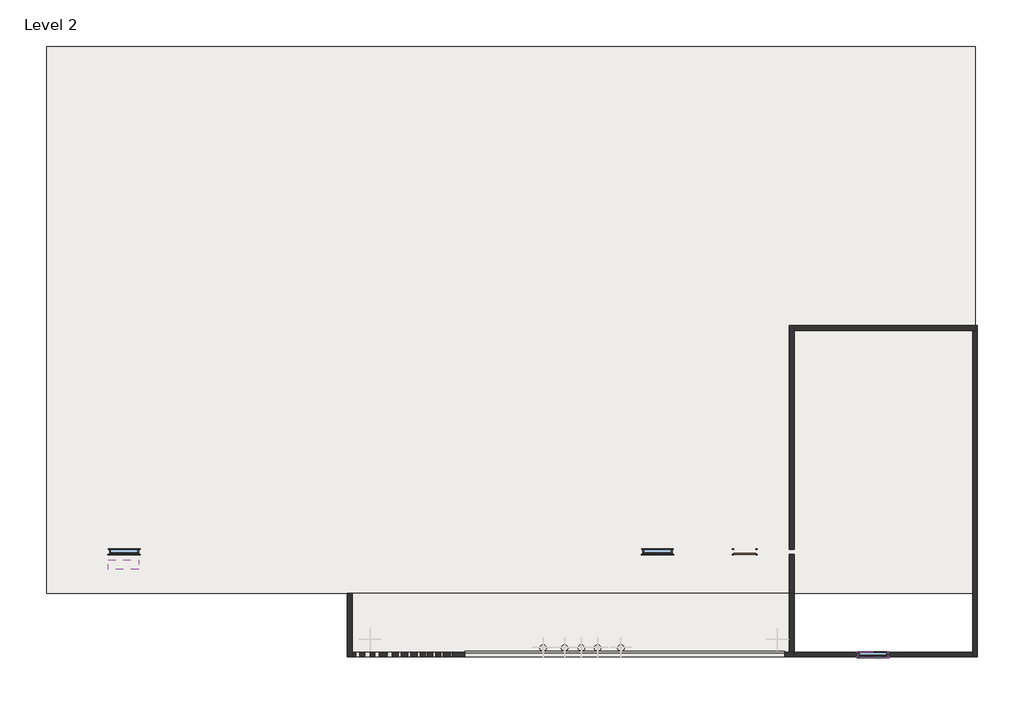
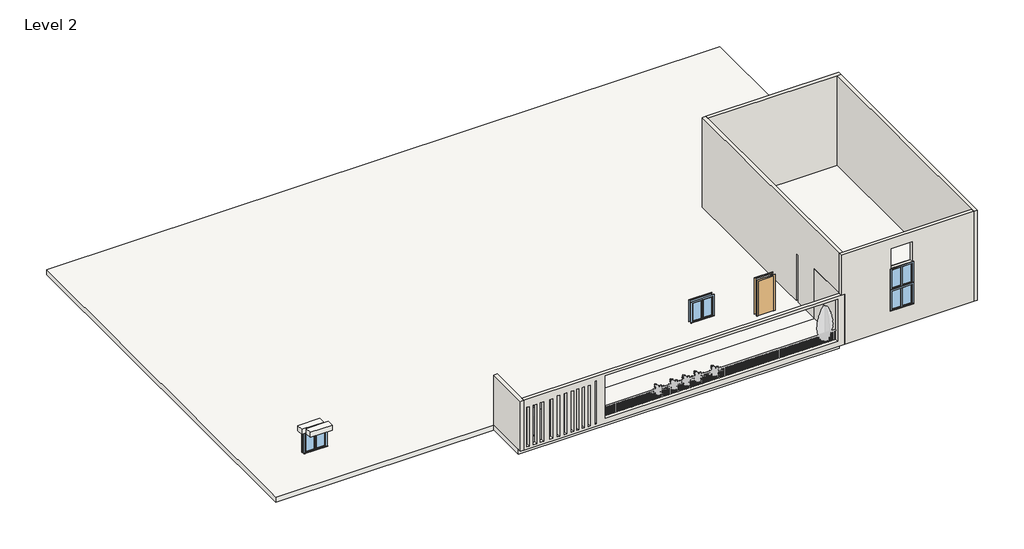
# One storey, part 1 of 2: 7 walls, 4 windows, 3 slabs, 1 door.
"""IFC4 building model written with IfcOpenShell, lengths in millimetres."""

from ifc_helpers import new_model, si_unit, frame, origin, place, context, project, spatial, polyline, outline, extrude, faceted_brep, transform, mapped, element, save
from components import door_54dd4da4, window_0862ab64

model = new_model("IFC4")

# Units and contexts
model_context = context("Model", 3, world=origin())
ifc_project = project(units=[si_unit("LENGTHUNIT", "METRE", prefix="MILLI")], contexts=[model_context])

# Site, building, storey
site = spatial("IfcSite", under=ifc_project)
building = spatial("IfcBuilding", under=site)
storey = spatial("IfcBuildingStorey", under=building, Name="Level 2", Elevation=3200.4)

# Door
placement = place(None, origin())
door_shape = door_54dd4da4(model_context)
element("IfcDoor", 1, ObjectType="Single-Flush : 36\" x 84\"", at=placement, inside=storey, context=model_context, shape_type="MappedRepresentation", body=[
    mapped(door_shape, transform((6933.8747398, -14818.870124, 3200.4), x_axis=(-1.0, 0.0, 0.0), y_axis=(0.0, -1.0, 0.0), z_axis=(0.0, 0.0, 1.0))),
])

# Slabs
element("IfcSlab", 2, ObjectType="Generic - 12\"", at=placement, inside=storey, context=model_context, shape_type="SweptSolid", body=[
    extrude(outline(polyline([(16585.8747398, 6378.5537948), (16585.8747398, -16555.9021378), (-22326.9252602, -16555.9021378), (-22326.9252602, 6378.5537948), (16585.8747398, 6378.5537948)])), frame((0.0, 0.0, 2895.6), z_axis=(0.0, 0.0, 1.0), x_axis=(1.0, 0.0, 0.0)), (0.0, 0.0, 1.0), 304.8),
])
element("IfcSlab", 3, ObjectType="Generic - 12\"", at=placement, inside=storey, context=model_context, shape_type="SweptSolid", body=[
    extrude(outline(polyline([(-18470.9809224, -15158.9638264), (-18470.9809224, -15539.9638264), (-19740.9809224, -15539.9638264), (-19740.9809224, -15158.9638264), (-18470.9809224, -15158.9638264)])), frame((0.0, 0.0, 5334.0), z_axis=(0.0, 0.0, 1.0), x_axis=(1.0, 0.0, 0.0)), (0.0, 0.0, 1.0), 304.8),
    extrude(outline(polyline([(-18710.9996532, -14717.270124), (-18710.9996532, -15098.270124), (-19980.9996532, -15098.270124), (-19980.9996532, -14717.270124), (-18710.9996532, -14717.270124)])), frame((0.0, 0.0, 5334.0), z_axis=(0.0, 0.0, 1.0), x_axis=(1.0, 0.0, 0.0)), (0.0, 0.0, 1.0), 304.8),
])
element("IfcSlab", 4, ObjectType="Generic - 12\"", at=placement, inside=storey, context=model_context, shape_type="SweptSolid", body=[
    extrude(outline(polyline([(8806.3760973, -16555.9021378), (8806.3760973, -19021.4462052), (-9727.8029191, -19021.4462052), (-9727.8029191, -16555.9021378), (8806.3760973, -16555.9021378)])), frame((0.0, 0.0, 2895.6), z_axis=(0.0, 0.0, 1.0), x_axis=(1.0, 0.0, 0.0)), (0.0, 0.0, 1.0), 304.8),
])

# Walls
element("IfcWall", 5, ObjectType="Generic - 8\"", at=placement, inside=storey, context=model_context, shape_type="Brep", body=[
    faceted_brep([(-9524.6029191, -19224.6462052, 3200.4), (-9524.6029191, -19021.4462052, 3200.4), (-9524.6029191, -16555.9021378, 3200.4), (-9524.6029191, -16555.9021378, 6248.4), (-9524.6029191, -19021.4462052, 6248.4), (-9524.6029191, -19224.6462052, 6248.4), (-9727.8029191, -19224.6462052, 3200.4), (-9727.8029191, -19224.6462052, 6248.4), (-9727.8029191, -16555.9021378, 6248.4), (-9727.8029191, -16555.9021378, 3200.4)], [[[0, 1, 2, 3, 4, 5]], [[6, 7, 8, 9]], [[2, 1, 0, 6, 9]], [[3, 2, 9, 8]], [[5, 4, 3, 8, 7]], [[0, 5, 7, 6]]]),
])
element("IfcWall", 6, ObjectType="Generic - 8\"", at=placement, inside=storey, context=model_context, shape_type="Brep", body=[
    faceted_brep([(9009.5760973, -19021.4462052, 3200.4), (8806.3760973, -19021.4462052, 3200.4), (-9524.6029191, -19021.4462052, 3200.4), (-9524.6029191, -19021.4462052, 6248.4), (8806.3760973, -19021.4462052, 6248.4), (9009.5760973, -19021.4462052, 6248.4), (8602.0331611, -19021.4462052, 6096.0), (-4809.1668389, -19021.4462052, 6096.0), (-4809.1668389, -19021.4462052, 3505.2), (8602.0331611, -19021.4462052, 3505.2), (-5331.1523958, -19021.4462052, 5990.1341587), (-5407.3523958, -19021.4462052, 5990.1341587), (-5407.3523958, -19021.4462052, 3348.5341587), (-5331.1523958, -19021.4462052, 3348.5341587), (-7464.3821742, -19021.4462052, 5843.7194015), (-7586.581963, -19021.4462052, 5843.7194015), (-7586.581963, -19021.4462052, 3348.5341587), (-7464.3821742, -19021.4462052, 3348.5341587), (-7057.0495448, -19021.4462052, 5843.7194015), (-7192.827088, -19021.4462052, 5843.7194015), (-7192.827088, -19021.4462052, 3348.5341587), (-7057.0495448, -19021.4462052, 3348.5341587), (-6656.5057926, -19021.4462052, 5843.7194015), (-6785.4944586, -19021.4462052, 5843.7194015), (-6785.4944586, -19021.4462052, 3348.5341587), (-6656.5057926, -19021.4462052, 3348.5341587), (-6364.5840749, -19021.4462052, 5843.7194015), (-6459.6283551, -19021.4462052, 5843.7194015), (-6459.6283551, -19021.4462052, 3348.5341587), (-6364.5840749, -19021.4462052, 3348.5341587), (-6025.1402171, -19021.4462052, 5843.7194015), (-6140.5511287, -19021.4462052, 5843.7194015), (-6140.5511287, -19021.4462052, 3348.5341587), (-6025.1402171, -19021.4462052, 3348.5341587), (-5699.2741136, -19021.4462052, 5843.7194015), (-5814.6850252, -19021.4462052, 5843.7194015), (-5814.6850252, -19021.4462052, 3348.5341587), (-5699.2741136, -19021.4462052, 3348.5341587), (-7844.559295, -19021.4462052, 5762.9412554), (-8041.4367325, -19021.4462052, 5762.9412554), (-8041.4367325, -19021.4462052, 3348.5341587), (-7844.559295, -19021.4462052, 3348.5341587), (-9209.1236034, -19021.4462052, 5762.9412554), (-9372.0566552, -19021.4462052, 5762.9412554), (-9372.0566552, -19021.4462052, 3348.5341587), (-9209.1236034, -19021.4462052, 3348.5341587), (-8770.6205738, -19021.4462052, 5762.9412554), (-8991.8795344, -19021.4462052, 5762.9412554), (-8991.8795344, -19021.4462052, 3348.5341587), (-8770.6205738, -19021.4462052, 3348.5341587), (-8380.8805903, -19021.4462052, 5762.9412554), (-8564.1802736, -19021.4462052, 5762.9412554), (-8564.1802736, -19021.4462052, 3348.5341587), (-8380.8805903, -19021.4462052, 3348.5341587), (9009.5760973, -19224.6462052, 3200.4), (9009.5760973, -19224.6462052, 6248.4), (8806.3760973, -19224.6462052, 6248.4), (-9524.6029191, -19224.6462052, 6248.4), (-9524.6029191, -19224.6462052, 3200.4), (8602.0331611, -19224.6462052, 6096.0), (8602.0331611, -19224.6462052, 3505.2), (-4809.1668389, -19224.6462052, 3505.2), (-4809.1668389, -19224.6462052, 6096.0), (-5331.1523958, -19224.6462052, 5990.1341587), (-5331.1523958, -19224.6462052, 3348.5341587), (-5407.3523958, -19224.6462052, 3348.5341587), (-5407.3523958, -19224.6462052, 5990.1341587), (-7464.3821742, -19224.6462052, 5843.7194015), (-7464.3821742, -19224.6462052, 3348.5341587), (-7586.581963, -19224.6462052, 3348.5341587), (-7586.581963, -19224.6462052, 5843.7194015), (-7057.0495448, -19224.6462052, 5843.7194015), (-7057.0495448, -19224.6462052, 3348.5341587), (-7192.827088, -19224.6462052, 3348.5341587), (-7192.827088, -19224.6462052, 5843.7194015), (-6656.5057926, -19224.6462052, 5843.7194015), (-6656.5057926, -19224.6462052, 3348.5341587), (-6785.4944586, -19224.6462052, 3348.5341587), (-6785.4944586, -19224.6462052, 5843.7194015), (-6364.5840749, -19224.6462052, 5843.7194015), (-6364.5840749, -19224.6462052, 3348.5341587), (-6459.6283551, -19224.6462052, 3348.5341587), (-6459.6283551, -19224.6462052, 5843.7194015), (-6025.1402171, -19224.6462052, 5843.7194015), (-6025.1402171, -19224.6462052, 3348.5341587), (-6140.5511287, -19224.6462052, 3348.5341587), (-6140.5511287, -19224.6462052, 5843.7194015), (-5699.2741136, -19224.6462052, 5843.7194015), (-5699.2741136, -19224.6462052, 3348.5341587), (-5814.6850252, -19224.6462052, 3348.5341587), (-5814.6850252, -19224.6462052, 5843.7194015), (-7844.559295, -19224.6462052, 5762.9412554), (-7844.559295, -19224.6462052, 3348.5341587), (-8041.4367325, -19224.6462052, 3348.5341587), (-8041.4367325, -19224.6462052, 5762.9412554), (-9209.1236034, -19224.6462052, 5762.9412554), (-9209.1236034, -19224.6462052, 3348.5341587), (-9372.0566552, -19224.6462052, 3348.5341587), (-9372.0566552, -19224.6462052, 5762.9412554), (-8770.6205738, -19224.6462052, 5762.9412554), (-8770.6205738, -19224.6462052, 3348.5341587), (-8991.8795344, -19224.6462052, 3348.5341587), (-8991.8795344, -19224.6462052, 5762.9412554), (-8380.8805903, -19224.6462052, 5762.9412554), (-8380.8805903, -19224.6462052, 3348.5341587), (-8564.1802736, -19224.6462052, 3348.5341587), (-8564.1802736, -19224.6462052, 5762.9412554)], [[[0, 1, 2, 3, 4, 5], [6, 7, 8, 9], [10, 11, 12, 13], [14, 15, 16, 17], [18, 19, 20, 21], [22, 23, 24, 25], [26, 27, 28, 29], [30, 31, 32, 33], [34, 35, 36, 37], [38, 39, 40, 41], [42, 43, 44, 45], [46, 47, 48, 49], [50, 51, 52, 53]], [[54, 55, 56, 57, 58], [59, 60, 61, 62], [63, 64, 65, 66], [67, 68, 69, 70], [71, 72, 73, 74], [75, 76, 77, 78], [79, 80, 81, 82], [83, 84, 85, 86], [87, 88, 89, 90], [91, 92, 93, 94], [95, 96, 97, 98], [99, 100, 101, 102], [103, 104, 105, 106]], [[0, 5, 55, 54]], [[3, 2, 58, 57]], [[2, 1, 0, 54, 58]], [[5, 4, 3, 57, 56, 55]], [[7, 6, 59, 62]], [[8, 7, 62, 61]], [[9, 8, 61, 60]], [[6, 9, 60, 59]], [[11, 10, 63, 66]], [[12, 11, 66, 65]], [[13, 12, 65, 64]], [[10, 13, 64, 63]], [[15, 14, 67, 70]], [[16, 15, 70, 69]], [[17, 16, 69, 68]], [[14, 17, 68, 67]], [[19, 18, 71, 74]], [[20, 19, 74, 73]], [[21, 20, 73, 72]], [[18, 21, 72, 71]], [[23, 22, 75, 78]], [[24, 23, 78, 77]], [[25, 24, 77, 76]], [[22, 25, 76, 75]], [[27, 26, 79, 82]], [[28, 27, 82, 81]], [[29, 28, 81, 80]], [[26, 29, 80, 79]], [[31, 30, 83, 86]], [[32, 31, 86, 85]], [[33, 32, 85, 84]], [[30, 33, 84, 83]], [[35, 34, 87, 90]], [[36, 35, 90, 89]], [[37, 36, 89, 88]], [[34, 37, 88, 87]], [[39, 38, 91, 94]], [[40, 39, 94, 93]], [[41, 40, 93, 92]], [[38, 41, 92, 91]], [[43, 42, 95, 98]], [[44, 43, 98, 97]], [[45, 44, 97, 96]], [[42, 45, 96, 95]], [[47, 46, 99, 102]], [[48, 47, 102, 101]], [[49, 48, 101, 100]], [[46, 49, 100, 99]], [[51, 50, 103, 106]], [[52, 51, 106, 105]], [[53, 52, 105, 104]], [[50, 53, 104, 103]]]),
])
element("IfcWall", 7, ObjectType="Generic - 8\"", at=placement, inside=storey, context=model_context, shape_type="SweptSolid", body=[
    extrude(outline(polyline([(8806.3760973, -19021.4462052), (8806.3760973, -16555.9021378), (9009.5760973, -16555.9021378), (9009.5760973, -19021.4462052), (8806.3760973, -19021.4462052)])), frame((0.0, 0.0, 3200.4), z_axis=(0.0, 0.0, 1.0), x_axis=(1.0, 0.0, 0.0)), (0.0, 0.0, 1.0), 3048.0),
])
element("IfcWall", 8, ObjectType="Generic - 8\"", at=placement, inside=storey, context=model_context, shape_type="Brep", body=[
    faceted_brep([(9009.5760973, -19224.6462052, 6248.4), (9009.5760973, -19224.6462052, 3200.4), (16484.2747398, -19224.6462052, 3200.4), (16484.2747398, -19224.6462052, 8686.8), (8806.3760973, -19224.6462052, 8686.8), (8806.3760973, -19224.6462052, 6248.4), (11701.9760973, -19224.6462052, 8090.2910199), (12921.1760973, -19224.6462052, 8090.2910199), (12921.1760973, -19224.6462052, 6871.0910199), (11701.9760973, -19224.6462052, 6871.0910199), (11701.9760973, -19224.6462052, 6806.5998731), (12921.1760973, -19224.6462052, 6806.5998731), (12921.1760973, -19224.6462052, 5587.3998731), (11701.9760973, -19224.6462052, 5587.3998731), (11701.9760973, -19224.6462052, 5520.3170072), (12921.1760973, -19224.6462052, 5520.3170072), (12921.1760973, -19224.6462052, 4301.1170072), (11701.9760973, -19224.6462052, 4301.1170072), (9009.5760973, -19021.4462052, 3200.4), (9009.5760973, -19021.4462052, 6248.4), (8806.3760973, -19021.4462052, 6248.4), (8806.3760973, -19021.4462052, 8686.8), (9009.5760973, -19021.4462052, 8686.8), (16484.2747398, -19021.4462052, 8686.8), (16484.2747398, -19021.4462052, 3200.4), (11701.9760973, -19021.4462052, 8090.2910199), (11701.9760973, -19021.4462052, 6871.0910199), (12921.1760973, -19021.4462052, 6871.0910199), (12921.1760973, -19021.4462052, 8090.2910199), (11701.9760973, -19021.4462052, 6806.5998731), (11701.9760973, -19021.4462052, 5587.3998731), (12921.1760973, -19021.4462052, 5587.3998731), (12921.1760973, -19021.4462052, 6806.5998731), (11701.9760973, -19021.4462052, 5520.3170072), (11701.9760973, -19021.4462052, 4301.1170072), (12921.1760973, -19021.4462052, 4301.1170072), (12921.1760973, -19021.4462052, 5520.3170072)], [[[0, 1, 2, 3, 4, 5], [6, 7, 8, 9], [10, 11, 12, 13], [14, 15, 16, 17]], [[18, 19, 20, 21, 22, 23, 24], [25, 26, 27, 28], [29, 30, 31, 32], [33, 34, 35, 36]], [[2, 1, 18, 24]], [[4, 3, 23, 22, 21]], [[3, 2, 24, 23]], [[5, 20, 19, 0]], [[0, 19, 18, 1]], [[5, 4, 21, 20]], [[26, 25, 6, 9]], [[27, 26, 9, 8]], [[28, 27, 8, 7]], [[25, 28, 7, 6]], [[30, 29, 10, 13]], [[31, 30, 13, 12]], [[32, 31, 12, 11]], [[29, 32, 11, 10]], [[34, 33, 14, 17]], [[35, 34, 17, 16]], [[36, 35, 16, 15]], [[33, 36, 15, 14]]]),
])
element("IfcWall", 9, ObjectType="Generic - 8\"", at=placement, inside=storey, context=model_context, shape_type="Brep", body=[
    faceted_brep([(8806.3760973, -19021.4462052, 8686.8), (8806.3760973, -5333.3996234, 8686.8), (8806.3760973, -5333.3996234, 3200.4), (8806.3760973, -14717.270124, 3200.4), (8806.3760973, -14717.270124, 6096.0), (8806.3760973, -14920.470124, 6096.0), (8806.3760973, -14920.470124, 3200.4), (8806.3760973, -19021.4462052, 3200.4), (8806.3760973, -19021.4462052, 6248.4), (9009.5760973, -5333.3996234, 8686.8), (9009.5760973, -5536.5996234, 8686.8), (9009.5760973, -19021.4462052, 8686.8), (9009.5760973, -19021.4462052, 6248.4), (9009.5760973, -19021.4462052, 3200.4), (9009.5760973, -14920.470124, 3200.4), (9009.5760973, -14920.470124, 6096.0), (9009.5760973, -14717.270124, 6096.0), (9009.5760973, -14717.270124, 3200.4), (9009.5760973, -5536.5996234, 3200.4), (9009.5760973, -5333.3996234, 3200.4)], [[[0, 1, 2, 3, 4, 5, 6, 7, 8]], [[9, 10, 11, 12, 13, 14, 15, 16, 17, 18, 19]], [[2, 19, 18, 17, 3]], [[13, 7, 6, 14]], [[1, 0, 11, 10, 9]], [[2, 1, 9, 19]], [[16, 4, 3, 17]], [[5, 15, 14, 6]], [[4, 16, 15, 5]], [[7, 13, 12, 11, 0, 8]]]),
])
element("IfcWall", 10, ObjectType="Generic - 8\"", at=placement, inside=storey, context=model_context, shape_type="Brep", body=[
    faceted_brep([(16687.4747398, -5333.3996234, 3200.4), (9009.5760973, -5333.3996234, 3200.4), (9009.5760973, -5333.3996234, 8686.8), (16687.4747398, -5333.3996234, 8686.8), (16687.4747398, -5536.5996234, 3200.4), (16687.4747398, -5536.5996234, 8686.8), (16484.2747398, -5536.5996234, 8686.8), (9009.5760973, -5536.5996234, 8686.8), (9009.5760973, -5536.5996234, 3200.4), (16484.2747398, -5536.5996234, 3200.4)], [[[0, 1, 2, 3]], [[4, 5, 6, 7, 8, 9]], [[1, 0, 4, 9, 8]], [[3, 2, 7, 6, 5]], [[0, 3, 5, 4]], [[2, 1, 8, 7]]]),
])
element("IfcWall", 11, ObjectType="Generic - 8\"", at=placement, inside=storey, context=model_context, shape_type="Brep", body=[
    faceted_brep([(16687.4747398, -19224.6462052, 3200.4), (16687.4747398, -5536.5996234, 3200.4), (16687.4747398, -5536.5996234, 8686.8), (16687.4747398, -19224.6462052, 8686.8), (16484.2747398, -19224.6462052, 3200.4), (16484.2747398, -19224.6462052, 8686.8), (16484.2747398, -19021.4462052, 8686.8), (16484.2747398, -5536.5996234, 8686.8), (16484.2747398, -5536.5996234, 3200.4), (16484.2747398, -19021.4462052, 3200.4)], [[[0, 1, 2, 3]], [[4, 5, 6, 7, 8, 9]], [[1, 0, 4, 9, 8]], [[3, 2, 7, 6, 5]], [[0, 3, 5, 4]], [[2, 1, 8, 7]]]),
])

# Windows
window_shape = window_0862ab64(model_context)
element("IfcWindow", 12, ObjectType="Casement Dbl with Trim : 48\" x 48\"", at=placement, inside=storey, context=model_context, shape_type="MappedRepresentation", body=[
    mapped(window_shape, transform((-19075.7252602, -14799.820124, 3051.5493756), x_axis=(-1.0, 0.0, 0.0), y_axis=(0.0, -1.0, 0.0), z_axis=(0.0, 0.0, 1.0))),
])
element("IfcWindow", 13, ObjectType="Casement Dbl with Trim : 48\" x 48\"", at=placement, inside=storey, context=model_context, shape_type="MappedRepresentation", body=[
    mapped(window_shape, transform((12311.5760973, -19103.9962052, 4672.9998731), x_axis=(-1.0, 0.0, 0.0), y_axis=(0.0, -1.0, 0.0), z_axis=(0.0, 0.0, 1.0))),
])
element("IfcWindow", 14, ObjectType="Casement Dbl with Trim : 48\" x 48\"", at=placement, inside=storey, context=model_context, shape_type="MappedRepresentation", body=[
    mapped(window_shape, transform((12311.5760973, -19103.9962052, 3386.7170072), x_axis=(-1.0, 0.0, 0.0), y_axis=(0.0, -1.0, 0.0), z_axis=(0.0, 0.0, 1.0))),
])
element("IfcWindow", 15, ObjectType="Casement Dbl with Trim : 48\" x 48\"", at=placement, inside=storey, context=model_context, shape_type="MappedRepresentation", body=[
    mapped(window_shape, transform((3276.2747398, -14799.820124, 3200.4), x_axis=(-1.0, 0.0, 0.0), y_axis=(0.0, -1.0, 0.0), z_axis=(0.0, 0.0, 1.0))),
])

save(model, "model.ifc")

# Revit data of these elements
# Type "Single-Flush : 36\" x 84\""
#   Type Mark = "1"
#   Construction Type Id = "MDOOR"
#   Assembly Code = "C1020"
#   Analytic Construction = "Metal"
#   Thickness = 0' - 2"
#   Heat Transfer Coefficient (U) = 0.651978 BTU/(h·ft²·°F)
#   Height = 7' - 0"
#   Trim Projection Ext = 0' - 1"
#   Trim Projection Int = 0' - 1"
#   Trim Width = 0' - 3"
#   Width = 3' - 0"
#   Define Thermal Properties by = 1
#   Door Material = Door - Panel
#   Frame Material = Door - Frame
#   Visual Light Transmittance = 0
#   Solar Heat Gain Coefficient = 0
#   Function = (empty or 0)
#   Wall Closure = (empty or 0)
# Type "Generic - 12\""
#   Assembly Code = "B1010"
#   Function = 0
#   Layers, outside or top first: 1' - 0" no material (function 1)
# Type "Generic - 8\""
#   Assembly Code = "B2010"
#   Layers, outside or top first: 0' - 8" no material (function 1)
# Type "Casement Dbl with Trim : 48\" x 48\""
#   Type Mark = "10"
#   Construction Type Id = "GSP4R"
#   Assembly Code = "B2020100"
#   Analytic Construction = "1/8 in Pilkington single glazing"
#   Visual Light Transmittance = 0.9
#   Solar Heat Gain Coefficient = 0.78
#   Heat Transfer Coefficient (U) = 0.6496 BTU/(h·ft²·°F)
#   Height = 4' - 0"
#   Default Sill Height = 3' - 0"
#   Trim Projection - Ext. = 0' - 0 1/2"
#   Trim Projection - Int. = 0' - 0 3/4"
#   Trim Width - Exterior = 0' - 3 1/2"
#   Trim Width - Interior = 0' - 3 1/2"
#   Width = 4' - 0"
#   Window Inset = 0' - 0 3/4"
#   Define Thermal Properties by = 1
#   Glass Pane Material = Glass
#   Sash Material = Glass
#   Trim Exterior Material = Glass, Clear Glazing
#   Trim Interior Material = Trim
#   Wall Closure = (empty or 0)
# Element 1 (IfcDoor, "Single-Flush : 36\" x 84\"")
#   Phase Created = New Construction
#   Materials on its faces: "Door - Frame", "Door - Panel"
# Elements 2, 4 (IfcSlab, "Generic - 12\"")
#   Height Offset From Level = 0' - 0"
#   Phase Created = New Construction
#   Materials on its faces: "Default Floor"
# Element 3 (IfcSlab, "Generic - 12\"")
#   Height Offset From Level = 8' - 0"
#   Phase Created = New Construction
#   Materials on its faces: "Default Floor"
# Elements 5, 6, 7 (IfcWall, "Generic - 8\"")
#   Top Offset = 0' - 0"
#   Base Offset = 0' - 0"
#   Unconnected Height = 10' - 0"
#   wall height = 10' - 0"
#   Phase Created = New Construction
#   Base Constraint = Level 2
#   Materials on its faces: "Default Wall"
# Elements 8, 9, 10, 11 (IfcWall, "Generic - 8\"")
#   Top Offset = 0' - 0"
#   Base Offset = 0' - 0"
#   Unconnected Height = 18' - 0"
#   wall height = 18' - 0"
#   Phase Created = New Construction
#   Base Constraint = Level 2
#   Materials on its faces: "Default Wall"
# Element 12 (IfcWindow, "Casement Dbl with Trim : 48\" x 48\"")
#   Mark = "1"
#   Phase Created = New Construction
#   Materials on its faces: "Glass", "Glass, Clear Glazing", "Trim"
# Element 13 (IfcWindow, "Casement Dbl with Trim : 48\" x 48\"")
#   Mark = "4"
#   Phase Created = New Construction
#   Materials on its faces: "Glass", "Glass, Clear Glazing", "Trim"
# Element 14 (IfcWindow, "Casement Dbl with Trim : 48\" x 48\"")
#   Mark = "5"
#   Phase Created = New Construction
#   Materials on its faces: "Glass", "Glass, Clear Glazing", "Trim"
# Element 15 (IfcWindow, "Casement Dbl with Trim : 48\" x 48\"")
#   Mark = "7"
#   Phase Created = New Construction
#   Materials on its faces: "Glass", "Glass, Clear Glazing", "Trim"
# Materials
#   "Door - Panel": class "Wood", colour RGB 210 159 95, transparency 0
#   "Door - Frame": colour RGB 118 70 51, transparency 0
#   "Glass": class "Glass", colour RGB 0 128 192, transparency 0.75, Description = "Soda Lime Glass", Cost = 0
#   "Glass, Clear Glazing": class "Glass", colour RGB 0 128 192, transparency 0.75, Description = "Clear glazing", Cost = 0
#   "Trim": class "Wood", colour RGB 224 178 126, transparency 0
#   "Default Floor": colour RGB 128 128 128, transparency 0
#   "Default Wall": colour RGB 128 128 128, transparency 0
